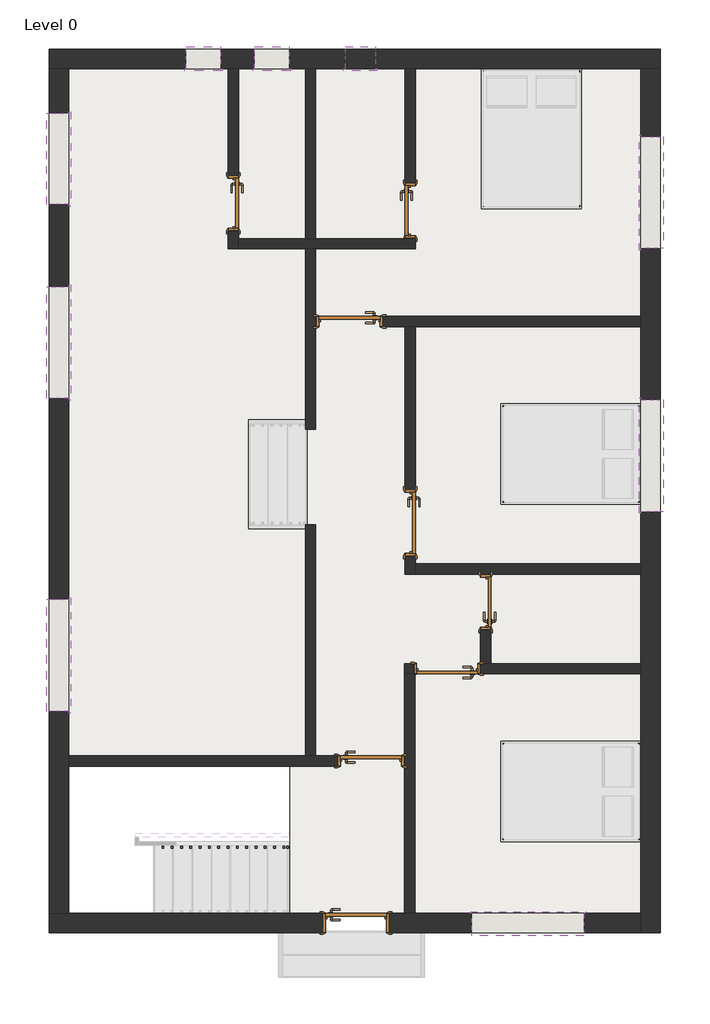
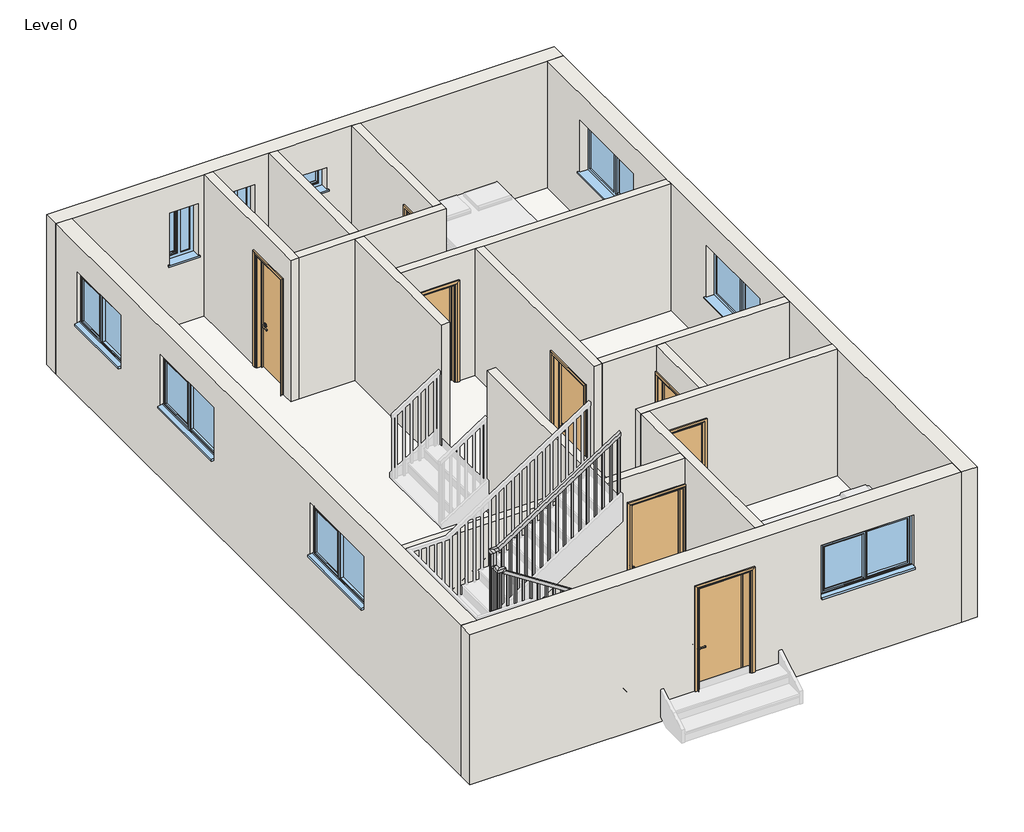
# One storey, part 1 of 2: 16 walls, 9 windows, 8 doors, 2 slabs, 1 railing.
"""IFC4 building model written with IfcOpenShell, lengths in millimetres."""

from ifc_helpers import new_model, si_unit, frame, origin, origin_with_axes, place, context, project, spatial, polyline, outline, extrude, faceted_brep, transform, mapped, element, save
from components import doors_intsgl_d1_661c03a1, doors_intsgl_d1_9c7e8c97, doors_intsgl_d1_8eed65bb, doors_intsgl_d2_f1ce814f, doors_intsgl_d2_e5ed4415, windows_dbl_plain_w1_1500_219ff321, windows_dbl_plain_w2_1220_793197e7, windows_dbl_plain_w3_460_956a2ca0, windows_sgl_plain_400mm_a5a4ca73

model = new_model("IFC4")

# Units and contexts
model_context = context("Model", 3, world=origin())
ifc_project = project(units=[si_unit("LENGTHUNIT", "METRE", prefix="MILLI")], contexts=[model_context])

# Site, building, storey
site = spatial("IfcSite", under=ifc_project)
building = spatial("IfcBuilding", under=site)
storey = spatial("IfcBuildingStorey", under=building, Name="Level 0", Elevation=0.0)

# Doors
placement = place(None, origin())
doors_intsgl_d1_shape = doors_intsgl_d1_661c03a1(model_context)
element("IfcDoor", 1, ObjectType="Doors_IntSgl : D1", at=placement, inside=storey, context=model_context, shape_type="MappedRepresentation", body=[
    mapped(doors_intsgl_d1_shape, transform((-4659.8904087, 8516.998858, 0.0), x_axis=(-1.0, 0.0, 0.0), y_axis=(0.0, -1.0, 0.0), z_axis=(0.0, 0.0, 1.0))),
])
doors_intsgl_d1_2_shape = doors_intsgl_d1_9c7e8c97(model_context)
element("IfcDoor", 2, ObjectType="Doors_IntSgl : D1", at=placement, inside=storey, context=model_context, shape_type="MappedRepresentation", body=[
    mapped(doors_intsgl_d1_2_shape, transform((-3844.8904087, 5816.998858, 0.0), x_axis=(0.0, -1.0, 0.0), y_axis=(1.0, 0.0, 0.0), z_axis=(0.0, 0.0, 1.0))),
])
element("IfcDoor", 3, ObjectType="Doors_IntSgl : D1", at=placement, inside=storey, context=model_context, shape_type="MappedRepresentation", body=[
    mapped(doors_intsgl_d1_2_shape, transform((-3349.8904087, 3856.998858, 0.0), x_axis=(-1.0, 0.0, 0.0), y_axis=(0.0, -1.0, 0.0), z_axis=(0.0, 0.0, 1.0))),
])
element("IfcDoor", 4, ObjectType="Doors_IntSgl : D1", at=placement, inside=storey, context=model_context, shape_type="MappedRepresentation", body=[
    mapped(doors_intsgl_d1_2_shape, transform((-4374.8904087, 2616.998858, 0.0), x_axis=(1.0, 0.0, 0.0), y_axis=(0.0, 1.0, 0.0), z_axis=(0.0, 0.0, 1.0))),
])
doors_intsgl_d1_3_shape = doors_intsgl_d1_8eed65bb(model_context)
element("IfcDoor", 5, ObjectType="Doors_IntSgl : D1", at=placement, inside=storey, context=model_context, shape_type="MappedRepresentation", body=[
    mapped(doors_intsgl_d1_3_shape, transform((-4574.8904087, 442.7642586, 0.0), x_axis=(1.0, 0.0, 0.0), y_axis=(0.0, 1.0, 0.0), z_axis=(0.0, 0.0, 1.0))),
])
doors_intsgl_d2_shape = doors_intsgl_d2_f1ce814f(model_context)
element("IfcDoor", 6, ObjectType="Doors_IntSgl : D2", at=placement, inside=storey, context=model_context, shape_type="MappedRepresentation", body=[
    mapped(doors_intsgl_d2_shape, transform((-3844.8904087, 10007.7642586, 0.0), x_axis=(0.0, -1.0, 0.0), y_axis=(1.0, 0.0, 0.0), z_axis=(0.0, 0.0, 1.0))),
])
element("IfcDoor", 7, ObjectType="Doors_IntSgl : D2", at=placement, inside=storey, context=model_context, shape_type="MappedRepresentation", body=[
    mapped(doors_intsgl_d2_shape, transform((-2829.8904087, 4751.998858, 0.0), x_axis=(0.0, 1.0, 0.0), y_axis=(-1.0, 0.0, 0.0), z_axis=(0.0, 0.0, 1.0))),
])
doors_intsgl_d2_2_shape = doors_intsgl_d2_e5ed4415(model_context)
element("IfcDoor", 8, ObjectType="Doors_IntSgl : D2", at=placement, inside=storey, context=model_context, shape_type="MappedRepresentation", body=[
    mapped(doors_intsgl_d2_2_shape, transform((-6224.8904087, 10107.7642586, 0.0), x_axis=(0.0, -1.0, 0.0), y_axis=(1.0, 0.0, 0.0), z_axis=(0.0, 0.0, 1.0))),
])

# Railing
element("IfcRailing", 9, ObjectType="1100mm", at=placement, inside=storey, context=model_context, shape_type="SolidModel", body=[
    faceted_brep([(-5481.4951322, 1436.1182736, 1266.6666667), (-5481.4951322, 1436.1182736, 1207.1072108), (-5481.4951322, 1486.1182736, 1207.1072108), (-5481.4951322, 1486.1182736, 1266.6666667), (-7466.8951322, 1436.1182736, 2551.7152104), (-7516.8951322, 1436.1182736, 2524.518214), (-7516.8951322, 1486.1182736, 2524.518214), (-7466.8951322, 1486.1182736, 2551.7152104), (-7466.8951322, 1436.1182736, 2600.0), (-7516.8951322, 1436.1182736, 2550.0), (-7516.8951322, 1486.1182736, 2550.0), (-7466.8951322, 1486.1182736, 2600.0), (-7591.8951322, 1436.1182736, 2600.0), (-7591.8951322, 1436.1182736, 2550.0), (-7541.8951322, 1486.1182736, 2550.0), (-7541.8951322, 1486.1182736, 2600.0), (-7591.8951322, 1561.1182736, 2600.0), (-7591.8951322, 1561.1182736, 2550.0), (-7541.8951322, 1561.1182736, 2550.0), (-7541.8951322, 1561.1182736, 2600.0), (-7591.8951322, 1571.9182736, 2600.0), (-7591.8951322, 1621.9182736, 2550.0), (-7541.8951322, 1621.9182736, 2550.0), (-7541.8951322, 1571.9182736, 2600.0), (-7591.8951322, 1571.9182736, 2814.9514563), (-7591.8951322, 1621.9182736, 2764.9514563), (-7541.8951322, 1621.9182736, 2764.9514563), (-7541.8951322, 1571.9182736, 2814.9514563), (-7591.8951322, 1696.9182736, 2814.9514563), (-7591.8951322, 1696.9182736, 2764.9514563), (-7541.8951322, 1646.9182736, 2764.9514563), (-7541.8951322, 1646.9182736, 2814.9514563), (-7466.8951322, 1696.9182736, 2814.9514563), (-7452.1257728, 1696.9182736, 2764.9514563), (-7452.1257728, 1646.9182736, 2764.9514563), (-7466.8951322, 1646.9182736, 2814.9514563), (-5481.4951322, 1696.9182736, 4100.0), (-5481.4951322, 1646.9182736, 4100.0), (-5481.4951322, 1646.9182736, 4040.4405441), (-5481.4951322, 1696.9182736, 4040.4405441)], [[[0, 1, 2, 3]], [[1, 0, 4, 5]], [[2, 1, 5, 6]], [[3, 2, 6, 7]], [[0, 3, 7, 4]], [[5, 4, 8, 9]], [[6, 5, 9, 10]], [[7, 6, 10, 11]], [[4, 7, 11, 8]], [[9, 8, 12, 13]], [[10, 9, 13, 14]], [[11, 10, 14, 15]], [[8, 11, 15, 12]], [[13, 12, 16, 17]], [[14, 13, 17, 18]], [[15, 14, 18, 19]], [[12, 15, 19, 16]], [[17, 16, 20, 21]], [[18, 17, 21, 22]], [[19, 18, 22, 23]], [[16, 19, 23, 20]], [[21, 20, 24, 25]], [[22, 21, 25, 26]], [[23, 22, 26, 27]], [[20, 23, 27, 24]], [[25, 24, 28, 29]], [[26, 25, 29, 30]], [[27, 26, 30, 31]], [[24, 27, 31, 28]], [[29, 28, 32, 33]], [[30, 29, 33, 34]], [[31, 30, 34, 35]], [[28, 31, 35, 32]], [[36, 37, 38, 39]], [[33, 32, 36, 39]], [[34, 33, 39, 38]], [[35, 34, 38, 37]], [[32, 35, 37, 36]]]),
    extrude(outline(polyline([(4017.5279227, -5516.8951322), (2833.3333333, -5516.8951322), (2833.3333333, -5491.8951322), (4033.7091525, -5491.8951322), (4017.5279227, -5516.8951322)])), frame((0.0, 1659.4182736, 0.0), z_axis=(0.0, 1.0, 0.0), x_axis=(0.0, 0.0, 1.0)), (0.0, 0.0, 1.0), 25.0),
    extrude(outline(polyline([(3936.6217739, -5641.8951322), (2833.3333333, -5641.8951322), (2833.3333333, -5616.8951322), (3952.8030036, -5616.8951322), (3936.6217739, -5641.8951322)])), frame((0.0, 1659.4182736, 0.0), z_axis=(0.0, 1.0, 0.0), x_axis=(0.0, 0.0, 1.0)), (0.0, 0.0, 1.0), 25.0),
    extrude(outline(polyline([(3855.715625, -5766.8951322), (2833.3333333, -5766.8951322), (2833.3333333, -5741.8951322), (3871.8968548, -5741.8951322), (3855.715625, -5766.8951322)])), frame((0.0, 1659.4182736, 0.0), z_axis=(0.0, 1.0, 0.0), x_axis=(0.0, 0.0, 1.0)), (0.0, 0.0, 1.0), 25.0),
    extrude(outline(polyline([(3774.8094761, -5891.8951322), (2666.6666667, -5891.8951322), (2666.6666667, -5866.8951322), (3790.9907059, -5866.8951322), (3774.8094761, -5891.8951322)])), frame((0.0, 1659.4182736, 0.0), z_axis=(0.0, 1.0, 0.0), x_axis=(0.0, 0.0, 1.0)), (0.0, 0.0, 1.0), 25.0),
    extrude(outline(polyline([(3693.9033273, -6016.8951322), (2500.0, -6016.8951322), (2500.0, -5991.8951322), (3710.084557, -5991.8951322), (3693.9033273, -6016.8951322)])), frame((0.0, 1659.4182736, 0.0), z_axis=(0.0, 1.0, 0.0), x_axis=(0.0, 0.0, 1.0)), (0.0, 0.0, 1.0), 25.0),
    extrude(outline(polyline([(3612.9971784, -6141.8951322), (2500.0, -6141.8951322), (2500.0, -6116.8951322), (3629.1784082, -6116.8951322), (3612.9971784, -6141.8951322)])), frame((0.0, 1659.4182736, 0.0), z_axis=(0.0, 1.0, 0.0), x_axis=(0.0, 0.0, 1.0)), (0.0, 0.0, 1.0), 25.0),
    extrude(outline(polyline([(3532.0910295, -6266.8951322), (2500.0, -6266.8951322), (2500.0, -6241.8951322), (3548.2722593, -6241.8951322), (3532.0910295, -6266.8951322)])), frame((0.0, 1659.4182736, 0.0), z_axis=(0.0, 1.0, 0.0), x_axis=(0.0, 0.0, 1.0)), (0.0, 0.0, 1.0), 25.0),
    extrude(outline(polyline([(3451.1848807, -6391.8951322), (2333.3333333, -6391.8951322), (2333.3333333, -6366.8951322), (3467.3661104, -6366.8951322), (3451.1848807, -6391.8951322)])), frame((0.0, 1659.4182736, 0.0), z_axis=(0.0, 1.0, 0.0), x_axis=(0.0, 0.0, 1.0)), (0.0, 0.0, 1.0), 25.0),
    extrude(outline(polyline([(3370.2787318, -6516.8951322), (2333.3333333, -6516.8951322), (2333.3333333, -6491.8951322), (3386.4599616, -6491.8951322), (3370.2787318, -6516.8951322)])), frame((0.0, 1659.4182736, 0.0), z_axis=(0.0, 1.0, 0.0), x_axis=(0.0, 0.0, 1.0)), (0.0, 0.0, 1.0), 25.0),
    extrude(outline(polyline([(3289.3725829, -6641.8951322), (2166.6666667, -6641.8951322), (2166.6666667, -6616.8951322), (3305.5538127, -6616.8951322), (3289.3725829, -6641.8951322)])), frame((0.0, 1659.4182736, 0.0), z_axis=(0.0, 1.0, 0.0), x_axis=(0.0, 0.0, 1.0)), (0.0, 0.0, 1.0), 25.0),
    extrude(outline(polyline([(3208.4664341, -6766.8951322), (2166.6666667, -6766.8951322), (2166.6666667, -6741.8951322), (3224.6476638, -6741.8951322), (3208.4664341, -6766.8951322)])), frame((0.0, 1659.4182736, 0.0), z_axis=(0.0, 1.0, 0.0), x_axis=(0.0, 0.0, 1.0)), (0.0, 0.0, 1.0), 25.0),
    extrude(outline(polyline([(3127.5602852, -6891.8951322), (2000.0, -6891.8951322), (2000.0, -6866.8951322), (3143.741515, -6866.8951322), (3127.5602852, -6891.8951322)])), frame((0.0, 1659.4182736, 0.0), z_axis=(0.0, 1.0, 0.0), x_axis=(0.0, 0.0, 1.0)), (0.0, 0.0, 1.0), 25.0),
    extrude(outline(polyline([(3046.6541363, -7016.8951322), (2000.0, -7016.8951322), (2000.0, -6991.8951322), (3062.8353661, -6991.8951322), (3046.6541363, -7016.8951322)])), frame((0.0, 1659.4182736, 0.0), z_axis=(0.0, 1.0, 0.0), x_axis=(0.0, 0.0, 1.0)), (0.0, 0.0, 1.0), 25.0),
    extrude(outline(polyline([(2965.7479875, -7141.8951322), (1833.3333333, -7141.8951322), (1833.3333333, -7116.8951322), (2981.9292172, -7116.8951322), (2965.7479875, -7141.8951322)])), frame((0.0, 1659.4182736, 0.0), z_axis=(0.0, 1.0, 0.0), x_axis=(0.0, 0.0, 1.0)), (0.0, 0.0, 1.0), 25.0),
    extrude(outline(polyline([(2884.8418386, -7266.8951322), (1833.3333333, -7266.8951322), (1833.3333333, -7241.8951322), (2901.0230684, -7241.8951322), (2884.8418386, -7266.8951322)])), frame((0.0, 1659.4182736, 0.0), z_axis=(0.0, 1.0, 0.0), x_axis=(0.0, 0.0, 1.0)), (0.0, 0.0, 1.0), 25.0),
    extrude(outline(polyline([(2803.9356897, -7391.8951322), (1666.6666667, -7391.8951322), (1666.6666667, -7366.8951322), (2820.1169195, -7366.8951322), (2803.9356897, -7391.8951322)])), frame((0.0, 1659.4182736, 0.0), z_axis=(0.0, 1.0, 0.0), x_axis=(0.0, 0.0, 1.0)), (0.0, 0.0, 1.0), 25.0),
    extrude(outline(polyline([(-7516.8951322, 1659.4182736), (-7516.8951322, 1684.4182736), (-7491.8951322, 1684.4182736), (-7491.8951322, 1659.4182736), (-7516.8951322, 1659.4182736)])), frame((0.0, 0.0, 1666.6666667), z_axis=(0.0, 0.0, 1.0), x_axis=(1.0, 0.0, 0.0)), (0.0, 0.0, 1.0), 1098.2847896),
    extrude(outline(polyline([(-7554.3951322, 1636.1182736), (-7579.3951322, 1636.1182736), (-7579.3951322, 1661.1182736), (-7554.3951322, 1661.1182736), (-7554.3951322, 1636.1182736)])), frame((0.0, 0.0, 1500.0), z_axis=(0.0, 0.0, 1.0), x_axis=(1.0, 0.0, 0.0)), (0.0, 0.0, 1.0), 1264.9514563),
    extrude(outline(polyline([(-7554.3951322, 1511.1182736), (-7579.3951322, 1511.1182736), (-7579.3951322, 1536.1182736), (-7554.3951322, 1536.1182736), (-7554.3951322, 1511.1182736)])), frame((0.0, 0.0, 1500.0), z_axis=(0.0, 0.0, 1.0), x_axis=(1.0, 0.0, 0.0)), (0.0, 0.0, 1.0), 1050.0),
    extrude(outline(polyline([(-7531.4951322, 1473.6182736), (-7531.4951322, 1448.6182736), (-7556.4951322, 1448.6182736), (-7556.4951322, 1473.6182736), (-7531.4951322, 1473.6182736)])), frame((0.0, 0.0, 1500.0), z_axis=(0.0, 0.0, 1.0), x_axis=(1.0, 0.0, 0.0)), (0.0, 0.0, 1.0), 1050.0),
    extrude(outline(polyline([(1333.3333333, -7406.4951322), (2453.0619033, -7406.4951322), (2469.2431331, -7431.4951322), (1333.3333333, -7431.4951322), (1333.3333333, -7406.4951322)])), frame((0.0, 1448.6182736, 0.0), z_axis=(0.0, 1.0, 0.0), x_axis=(0.0, 0.0, 1.0)), (0.0, 0.0, 1.0), 25.0),
    extrude(outline(polyline([(1333.3333333, -7281.4951322), (2372.1557544, -7281.4951322), (2388.3369842, -7306.4951322), (1333.3333333, -7306.4951322), (1333.3333333, -7281.4951322)])), frame((0.0, 1448.6182736, 0.0), z_axis=(0.0, 1.0, 0.0), x_axis=(0.0, 0.0, 1.0)), (0.0, 0.0, 1.0), 25.0),
    extrude(outline(polyline([(1166.6666667, -7156.4951322), (2291.2496056, -7156.4951322), (2307.4308354, -7181.4951322), (1166.6666667, -7181.4951322), (1166.6666667, -7156.4951322)])), frame((0.0, 1448.6182736, 0.0), z_axis=(0.0, 1.0, 0.0), x_axis=(0.0, 0.0, 1.0)), (0.0, 0.0, 1.0), 25.0),
    extrude(outline(polyline([(1166.6666667, -7031.4951322), (2210.3434567, -7031.4951322), (2226.5246865, -7056.4951322), (1166.6666667, -7056.4951322), (1166.6666667, -7031.4951322)])), frame((0.0, 1448.6182736, 0.0), z_axis=(0.0, 1.0, 0.0), x_axis=(0.0, 0.0, 1.0)), (0.0, 0.0, 1.0), 25.0),
    extrude(outline(polyline([(1000.0, -6906.4951322), (2129.4373078, -6906.4951322), (2145.6185376, -6931.4951322), (1000.0, -6931.4951322), (1000.0, -6906.4951322)])), frame((0.0, 1448.6182736, 0.0), z_axis=(0.0, 1.0, 0.0), x_axis=(0.0, 0.0, 1.0)), (0.0, 0.0, 1.0), 25.0),
    extrude(outline(polyline([(1000.0, -6781.4951322), (2048.531159, -6781.4951322), (2064.7123888, -6806.4951322), (1000.0, -6806.4951322), (1000.0, -6781.4951322)])), frame((0.0, 1448.6182736, 0.0), z_axis=(0.0, 1.0, 0.0), x_axis=(0.0, 0.0, 1.0)), (0.0, 0.0, 1.0), 25.0),
    extrude(outline(polyline([(833.3333333, -6656.4951322), (1967.6250101, -6656.4951322), (1983.8062399, -6681.4951322), (833.3333333, -6681.4951322), (833.3333333, -6656.4951322)])), frame((0.0, 1448.6182736, 0.0), z_axis=(0.0, 1.0, 0.0), x_axis=(0.0, 0.0, 1.0)), (0.0, 0.0, 1.0), 25.0),
    extrude(outline(polyline([(833.3333333, -6531.4951322), (1886.7188612, -6531.4951322), (1902.900091, -6556.4951322), (833.3333333, -6556.4951322), (833.3333333, -6531.4951322)])), frame((0.0, 1448.6182736, 0.0), z_axis=(0.0, 1.0, 0.0), x_axis=(0.0, 0.0, 1.0)), (0.0, 0.0, 1.0), 25.0),
    extrude(outline(polyline([(666.6666667, -6406.4951322), (1805.8127124, -6406.4951322), (1821.9939422, -6431.4951322), (666.6666667, -6431.4951322), (666.6666667, -6406.4951322)])), frame((0.0, 1448.6182736, 0.0), z_axis=(0.0, 1.0, 0.0), x_axis=(0.0, 0.0, 1.0)), (0.0, 0.0, 1.0), 25.0),
    extrude(outline(polyline([(666.6666667, -6281.4951322), (1724.9065635, -6281.4951322), (1741.0877933, -6306.4951322), (666.6666667, -6306.4951322), (666.6666667, -6281.4951322)])), frame((0.0, 1448.6182736, 0.0), z_axis=(0.0, 1.0, 0.0), x_axis=(0.0, 0.0, 1.0)), (0.0, 0.0, 1.0), 25.0),
    extrude(outline(polyline([(500.0, -6156.4951322), (1644.0004146, -6156.4951322), (1660.1816444, -6181.4951322), (500.0, -6181.4951322), (500.0, -6156.4951322)])), frame((0.0, 1448.6182736, 0.0), z_axis=(0.0, 1.0, 0.0), x_axis=(0.0, 0.0, 1.0)), (0.0, 0.0, 1.0), 25.0),
    extrude(outline(polyline([(500.0, -6031.4951322), (1563.0942658, -6031.4951322), (1579.2754955, -6056.4951322), (500.0, -6056.4951322), (500.0, -6031.4951322)])), frame((0.0, 1448.6182736, 0.0), z_axis=(0.0, 1.0, 0.0), x_axis=(0.0, 0.0, 1.0)), (0.0, 0.0, 1.0), 25.0),
    extrude(outline(polyline([(333.3333333, -5906.4951322), (1482.1881169, -5906.4951322), (1498.3693467, -5931.4951322), (333.3333333, -5931.4951322), (333.3333333, -5906.4951322)])), frame((0.0, 1448.6182736, 0.0), z_axis=(0.0, 1.0, 0.0), x_axis=(0.0, 0.0, 1.0)), (0.0, 0.0, 1.0), 25.0),
    extrude(outline(polyline([(333.3333333, -5781.4951322), (1401.281968, -5781.4951322), (1417.4631978, -5806.4951322), (333.3333333, -5806.4951322), (333.3333333, -5781.4951322)])), frame((0.0, 1448.6182736, 0.0), z_axis=(0.0, 1.0, 0.0), x_axis=(0.0, 0.0, 1.0)), (0.0, 0.0, 1.0), 25.0),
    extrude(outline(polyline([(166.6666667, -5656.4951322), (1320.3758192, -5656.4951322), (1336.5570489, -5681.4951322), (166.6666667, -5681.4951322), (166.6666667, -5656.4951322)])), frame((0.0, 1448.6182736, 0.0), z_axis=(0.0, 1.0, 0.0), x_axis=(0.0, 0.0, 1.0)), (0.0, 0.0, 1.0), 25.0),
    extrude(outline(polyline([(166.6666667, -5531.4951322), (1239.4696703, -5531.4951322), (1255.6509001, -5556.4951322), (166.6666667, -5556.4951322), (166.6666667, -5531.4951322)])), frame((0.0, 1448.6182736, 0.0), z_axis=(0.0, 1.0, 0.0), x_axis=(0.0, 0.0, 1.0)), (0.0, 0.0, 1.0), 25.0),
    extrude(outline(polyline([(-7554.3951322, 1659.4182736), (-7579.3951322, 1659.4182736), (-7579.3951322, 1684.4182736), (-7554.3951322, 1684.4182736), (-7554.3951322, 1659.4182736)])), frame((0.0, 0.0, 1500.0), z_axis=(0.0, 0.0, 1.0), x_axis=(1.0, 0.0, 0.0)), (0.0, 0.0, 1.0), 1264.9514563),
    extrude(outline(polyline([(-7554.3951322, 1473.6182736), (-7554.3951322, 1448.6182736), (-7579.3951322, 1448.6182736), (-7579.3951322, 1473.6182736), (-7554.3951322, 1473.6182736)])), frame((0.0, 0.0, 1500.0), z_axis=(0.0, 0.0, 1.0), x_axis=(1.0, 0.0, 0.0)), (0.0, 0.0, 1.0), 1050.0),
    extrude(outline(polyline([(4024.2593143, -5506.4951322), (2833.3333333, -5506.4951322), (2833.3333333, -5481.4951322), (4040.4405441, -5481.4951322), (4024.2593143, -5506.4951322)])), frame((0.0, 1659.4182736, 0.0), z_axis=(0.0, 1.0, 0.0), x_axis=(0.0, 0.0, 1.0)), (0.0, 0.0, 1.0), 25.0),
    extrude(outline(polyline([(166.6666667, -5481.4951322), (1207.1072108, -5481.4951322), (1223.2884405, -5506.4951322), (166.6666667, -5506.4951322), (166.6666667, -5481.4951322)])), frame((0.0, 1448.6182736, 0.0), z_axis=(0.0, 1.0, 0.0), x_axis=(0.0, 0.0, 1.0)), (0.0, 0.0, 1.0), 25.0),
])

# Slabs
element("IfcSlab", 10, ObjectType="FLOOR 150MM", at=placement, inside=storey, context=model_context, shape_type="SweptSolid", body=[
    extrude(outline(polyline([(-744.8904087, 11912.7642586), (-744.8904087, 572.7642586), (-5458.9951322, 572.7642586), (-5458.9951322, 2546.998858), (-5254.8904087, 2546.998858), (-5254.8904087, 11912.7642586), (-744.8904087, 11912.7642586)])), frame((0.0, 0.0, 250.0), z_axis=(0.0, 0.0, 1.0), x_axis=(1.0, 0.0, 0.0)), (0.0, 0.0, 1.0), 150.0),
])
element("IfcSlab", 11, ObjectType="FLOOR 150MM", at=placement, inside=storey, context=model_context, shape_type="SweptSolid", body=[
    extrude(outline(polyline([(-5254.8904087, 11912.7642586), (-5254.8904087, 2686.998858), (-8434.8904087, 2686.998858), (-8434.8904087, 11912.7642586), (-5254.8904087, 11912.7642586)])), origin_with_axes(), (0.0, 0.0, 1.0), 150.0),
])

# Walls
element("IfcWall", 12, at=placement, inside=storey, context=model_context, shape_type="Brep", body=[
    faceted_brep([(-8694.8904087, 11912.7642586, 0.0), (-8434.8904087, 11912.7642586, 0.0), (-6294.8904087, 11912.7642586, 0.0), (-6154.8904087, 11912.7642586, 0.0), (-5254.8904087, 11912.7642586, 0.0), (-5114.8904087, 11912.7642586, 0.0), (-3914.8904087, 11912.7642586, 0.0), (-3774.8904087, 11912.7642586, 0.0), (-744.8904087, 11912.7642586, 0.0), (-484.8904087, 11912.7642586, 0.0), (-484.8904087, 11912.7642586, 2570.0), (-744.8904087, 11912.7642586, 2570.0), (-3774.8904087, 11912.7642586, 2570.0), (-3914.8904087, 11912.7642586, 2570.0), (-5114.8904087, 11912.7642586, 2570.0), (-5254.8904087, 11912.7642586, 2570.0), (-6154.8904087, 11912.7642586, 2570.0), (-6294.8904087, 11912.7642586, 2570.0), (-8434.8904087, 11912.7642586, 2570.0), (-8694.8904087, 11912.7642586, 2570.0), (-6394.8904087, 11912.7642586, 2110.0), (-6394.8904087, 11912.7642586, 1200.0), (-6854.8904087, 11912.7642586, 1200.0), (-6854.8904087, 11912.7642586, 2110.0), (-5474.8904087, 11912.7642586, 2110.0), (-5474.8904087, 11912.7642586, 1200.0), (-5934.8904087, 11912.7642586, 1200.0), (-5934.8904087, 11912.7642586, 2110.0), (-4314.8904087, 11912.7642586, 2000.0), (-4314.8904087, 11912.7642586, 1600.0), (-4714.8904087, 11912.7642586, 1600.0), (-4714.8904087, 11912.7642586, 2000.0), (-484.8904087, 12172.7642586, 0.0), (-8694.8904087, 12172.7642586, 0.0), (-8694.8904087, 12172.7642586, 2570.0), (-484.8904087, 12172.7642586, 2570.0), (-6394.8904087, 12172.7642586, 1200.0), (-6394.8904087, 12172.7642586, 2110.0), (-6854.8904087, 12172.7642586, 2110.0), (-6854.8904087, 12172.7642586, 1200.0), (-5474.8904087, 12172.7642586, 1200.0), (-5474.8904087, 12172.7642586, 2110.0), (-5934.8904087, 12172.7642586, 2110.0), (-5934.8904087, 12172.7642586, 1200.0), (-4314.8904087, 12172.7642586, 1600.0), (-4314.8904087, 12172.7642586, 2000.0), (-4714.8904087, 12172.7642586, 2000.0), (-4714.8904087, 12172.7642586, 1600.0)], [[[0, 1, 2, 3, 4, 5, 6, 7, 8, 9, 10, 11, 12, 13, 14, 15, 16, 17, 18, 19], [20, 21, 22, 23], [24, 25, 26, 27], [28, 29, 30, 31]], [[32, 33, 34, 35], [36, 37, 38, 39], [40, 41, 42, 43], [44, 45, 46, 47]], [[9, 8, 7, 6, 5, 4, 3, 2, 1, 0, 33, 32]], [[10, 9, 32, 35]], [[0, 19, 34, 33]], [[19, 18, 17, 16, 15, 14, 13, 12, 11, 10, 35, 34]], [[21, 20, 37, 36]], [[22, 21, 36, 39]], [[23, 22, 39, 38]], [[20, 23, 38, 37]], [[25, 24, 41, 40]], [[26, 25, 40, 43]], [[27, 26, 43, 42]], [[24, 27, 42, 41]], [[28, 45, 44, 29]], [[29, 44, 47, 30]], [[30, 47, 46, 31]], [[45, 28, 31, 46]]]),
])
element("IfcWall", 13, at=placement, inside=storey, context=model_context, shape_type="Brep", body=[
    faceted_brep([(-744.8904087, 11912.7642586, 0.0), (-744.8904087, 8586.998858, 0.0), (-744.8904087, 8446.998858, 0.0), (-744.8904087, 5266.998858, 0.0), (-744.8904087, 5126.998858, 0.0), (-744.8904087, 3926.998858, 0.0), (-744.8904087, 3786.998858, 0.0), (-744.8904087, 572.7642586, 0.0), (-744.8904087, 312.7642586, 0.0), (-744.8904087, 312.7642586, 2570.0), (-744.8904087, 572.7642586, 2570.0), (-744.8904087, 3786.998858, 2570.0), (-744.8904087, 3926.998858, 2570.0), (-744.8904087, 5126.998858, 2570.0), (-744.8904087, 5266.998858, 2570.0), (-744.8904087, 8446.998858, 2570.0), (-744.8904087, 8586.998858, 2570.0), (-744.8904087, 11912.7642586, 2570.0), (-744.8904087, 10999.8815583, 2110.0), (-744.8904087, 9499.8815583, 2110.0), (-744.8904087, 9499.8815583, 1200.0), (-744.8904087, 10999.8815583, 1200.0), (-744.8904087, 7466.998858, 2110.0), (-744.8904087, 5966.998858, 2110.0), (-744.8904087, 5966.998858, 1200.0), (-744.8904087, 7466.998858, 1200.0), (-484.8904087, 11912.7642586, 0.0), (-484.8904087, 11912.7642586, 2570.0), (-484.8904087, 312.7642586, 2570.0), (-484.8904087, 312.7642586, 0.0), (-484.8904087, 10999.8815583, 2110.0), (-484.8904087, 10999.8815583, 1200.0), (-484.8904087, 9499.8815583, 1200.0), (-484.8904087, 9499.8815583, 2110.0), (-484.8904087, 7466.998858, 2110.0), (-484.8904087, 7466.998858, 1200.0), (-484.8904087, 5966.998858, 1200.0), (-484.8904087, 5966.998858, 2110.0)], [[[0, 1, 2, 3, 4, 5, 6, 7, 8, 9, 10, 11, 12, 13, 14, 15, 16, 17], [18, 19, 20, 21], [22, 23, 24, 25]], [[26, 27, 28, 29], [30, 31, 32, 33], [34, 35, 36, 37]], [[8, 7, 6, 5, 4, 3, 2, 1, 0, 26, 29]], [[0, 17, 27, 26]], [[9, 8, 29, 28]], [[17, 16, 15, 14, 13, 12, 11, 10, 9, 28, 27]], [[31, 30, 18, 21]], [[32, 31, 21, 20]], [[33, 32, 20, 19]], [[30, 33, 19, 18]], [[35, 34, 22, 25]], [[36, 35, 25, 24]], [[37, 36, 24, 23]], [[34, 37, 23, 22]]]),
])
element("IfcWall", 14, at=placement, inside=storey, context=model_context, shape_type="Brep", body=[
    faceted_brep([(-744.8904087, 572.7642586, 2570.0), (-744.8904087, 572.7642586, 0.0), (-3784.8904087, 572.7642586, 0.0), (-3924.8904087, 572.7642586, 0.0), (-4124.8904087, 572.7642586, 0.0), (-4124.8904087, 572.7642586, 2100.0), (-5024.8904087, 572.7642586, 2100.0), (-5024.8904087, 572.7642586, 0.0), (-8434.8904087, 572.7642586, 0.0), (-8694.8904087, 572.7642586, 0.0), (-8694.8904087, 572.7642586, 2570.0), (-8434.8904087, 572.7642586, 2570.0), (-3924.8904087, 572.7642586, 2570.0), (-3784.8904087, 572.7642586, 2570.0), (-1514.8904087, 572.7642586, 2110.0), (-3014.8904087, 572.7642586, 2110.0), (-3014.8904087, 572.7642586, 1200.0), (-1514.8904087, 572.7642586, 1200.0), (-744.8904087, 312.7642586, 0.0), (-744.8904087, 312.7642586, 2570.0), (-8694.8904087, 312.7642586, 2570.0), (-8694.8904087, 312.7642586, 0.0), (-5024.8904087, 312.7642586, 0.0), (-5024.8904087, 312.7642586, 2100.0), (-4124.8904087, 312.7642586, 2100.0), (-4124.8904087, 312.7642586, 0.0), (-1514.8904087, 312.7642586, 2110.0), (-1514.8904087, 312.7642586, 1200.0), (-3014.8904087, 312.7642586, 1200.0), (-3014.8904087, 312.7642586, 2110.0)], [[[0, 1, 2, 3, 4, 5, 6, 7, 8, 9, 10, 11, 12, 13], [14, 15, 16, 17]], [[18, 19, 20, 21, 22, 23, 24, 25], [26, 27, 28, 29]], [[1, 18, 25, 4, 3, 2]], [[21, 9, 8, 7, 22]], [[1, 0, 19, 18]], [[10, 9, 21, 20]], [[24, 5, 4, 25]], [[5, 24, 23, 6]], [[6, 23, 22, 7]], [[0, 13, 12, 11, 10, 20, 19]], [[27, 26, 14, 17]], [[28, 27, 17, 16]], [[29, 28, 16, 15]], [[26, 29, 15, 14]]]),
])
element("IfcWall", 15, at=placement, inside=storey, context=model_context, shape_type="Brep", body=[
    faceted_brep([(-8434.8904087, 572.7642586, 0.0), (-8434.8904087, 2546.998858, 0.0), (-8434.8904087, 2686.998858, 0.0), (-8434.8904087, 11912.7642586, 0.0), (-8434.8904087, 11912.7642586, 2570.0), (-8434.8904087, 2686.998858, 2570.0), (-8434.8904087, 2546.998858, 2570.0), (-8434.8904087, 572.7642586, 2570.0), (-8434.8904087, 3286.998858, 2110.0), (-8434.8904087, 4786.998858, 2110.0), (-8434.8904087, 4786.998858, 1200.0), (-8434.8904087, 3286.998858, 1200.0), (-8434.8904087, 7486.998858, 2110.0), (-8434.8904087, 8986.998858, 2110.0), (-8434.8904087, 8986.998858, 1200.0), (-8434.8904087, 7486.998858, 1200.0), (-8434.8904087, 10092.7642586, 2110.0), (-8434.8904087, 11312.7642586, 2110.0), (-8434.8904087, 11312.7642586, 1200.0), (-8434.8904087, 10092.7642586, 1200.0), (-8694.8904087, 572.7642586, 0.0), (-8694.8904087, 572.7642586, 2570.0), (-8694.8904087, 11912.7642586, 2570.0), (-8694.8904087, 11912.7642586, 0.0), (-8694.8904087, 3286.998858, 2110.0), (-8694.8904087, 3286.998858, 1200.0), (-8694.8904087, 4786.998858, 1200.0), (-8694.8904087, 4786.998858, 2110.0), (-8694.8904087, 7486.998858, 2110.0), (-8694.8904087, 7486.998858, 1200.0), (-8694.8904087, 8986.998858, 1200.0), (-8694.8904087, 8986.998858, 2110.0), (-8694.8904087, 10092.7642586, 2110.0), (-8694.8904087, 10092.7642586, 1200.0), (-8694.8904087, 11312.7642586, 1200.0), (-8694.8904087, 11312.7642586, 2110.0)], [[[0, 1, 2, 3, 4, 5, 6, 7], [8, 9, 10, 11], [12, 13, 14, 15], [16, 17, 18, 19]], [[20, 21, 22, 23], [24, 25, 26, 27], [28, 29, 30, 31], [32, 33, 34, 35]], [[3, 2, 1, 0, 20, 23]], [[4, 3, 23, 22]], [[0, 7, 21, 20]], [[7, 6, 5, 4, 22, 21]], [[25, 24, 8, 11]], [[26, 25, 11, 10]], [[27, 26, 10, 9]], [[24, 27, 9, 8]], [[29, 28, 12, 15]], [[30, 29, 15, 14]], [[31, 30, 14, 13]], [[28, 31, 13, 12]], [[33, 32, 16, 19]], [[34, 33, 19, 18]], [[35, 34, 18, 17]], [[32, 35, 17, 16]]]),
])
element("IfcWall", 16, ObjectType="140MM INNER WALL", at=placement, inside=storey, context=model_context, shape_type="Brep", body=[
    faceted_brep([(-6294.8904087, 11912.7642586, 2570.0), (-6294.8904087, 11912.7642586, 0.0), (-6294.8904087, 10482.7642586, 0.0), (-6294.8904087, 10482.7642586, 2100.0), (-6294.8904087, 9732.7642586, 2100.0), (-6294.8904087, 9732.7642586, 0.0), (-6294.8904087, 9492.7642586, 0.0), (-6294.8904087, 9492.7642586, 2570.0), (-6154.8904087, 11912.7642586, 0.0), (-6154.8904087, 11912.7642586, 2570.0), (-6154.8904087, 9632.7642586, 2570.0), (-6154.8904087, 9492.7642586, 2570.0), (-6154.8904087, 9492.7642586, 0.0), (-6154.8904087, 9632.7642586, 0.0), (-6154.8904087, 9732.7642586, 0.0), (-6154.8904087, 9732.7642586, 2100.0), (-6154.8904087, 10482.7642586, 2100.0), (-6154.8904087, 10482.7642586, 0.0)], [[[0, 1, 2, 3, 4, 5, 6, 7]], [[8, 9, 10, 11, 12, 13, 14, 15, 16, 17]], [[1, 8, 17, 2]], [[12, 6, 5, 14, 13]], [[1, 0, 9, 8]], [[7, 6, 12, 11]], [[4, 15, 14, 5]], [[15, 4, 3, 16]], [[16, 3, 2, 17]], [[0, 7, 11, 10, 9]]]),
])
element("IfcWall", 17, ObjectType="140MM INNER WALL", at=placement, inside=storey, context=model_context, shape_type="Brep", body=[
    faceted_brep([(-6154.8904087, 9492.7642586, 0.0), (-5254.8904087, 9492.7642586, 0.0), (-5114.8904087, 9492.7642586, 0.0), (-3774.8904087, 9492.7642586, 0.0), (-3774.8904087, 9492.7642586, 2570.0), (-5114.8904087, 9492.7642586, 2570.0), (-5254.8904087, 9492.7642586, 2570.0), (-6154.8904087, 9492.7642586, 2570.0), (-6154.8904087, 9632.7642586, 0.0), (-6154.8904087, 9632.7642586, 2570.0), (-5254.8904087, 9632.7642586, 2570.0), (-5114.8904087, 9632.7642586, 2570.0), (-3914.8904087, 9632.7642586, 2570.0), (-3774.8904087, 9632.7642586, 2570.0), (-3774.8904087, 9632.7642586, 2100.0), (-3774.8904087, 9632.7642586, 0.0), (-5114.8904087, 9632.7642586, 0.0), (-5254.8904087, 9632.7642586, 0.0)], [[[0, 1, 2, 3, 4, 5, 6, 7]], [[8, 9, 10, 11, 12, 13, 14, 15, 16, 17]], [[3, 2, 1, 0, 8, 17, 16, 15]], [[0, 7, 9, 8]], [[4, 3, 15, 14, 13]], [[7, 6, 5, 4, 13, 12, 11, 10, 9]]]),
])
element("IfcWall", 18, ObjectType="140MM INNER WALL", at=placement, inside=storey, context=model_context, shape_type="SweptSolid", body=[
    extrude(outline(polyline([(11912.7642586, 2570.0), (11912.7642586, 0.0), (10382.7642586, 0.0), (10382.7642586, 2100.0), (9632.7642586, 2100.0), (9632.7642586, 2570.0), (11912.7642586, 2570.0)])), frame((-3914.8904087, 0.0, 0.0), z_axis=(1.0, 0.0, 0.0), x_axis=(0.0, 1.0, 0.0)), (0.0, 0.0, 1.0), 140.0),
])
element("IfcWall", 19, ObjectType="140MM INNER WALL", at=placement, inside=storey, context=model_context, shape_type="Brep", body=[
    faceted_brep([(-5254.8904087, 7072.7642586, 0.0), (-5254.8904087, 7072.7642586, 2570.0), (-5254.8904087, 9492.7642586, 2570.0), (-5254.8904087, 9492.7642586, 0.0), (-5114.8904087, 7072.7642586, 2570.0), (-5114.8904087, 7072.7642586, 0.0), (-5114.8904087, 8446.998858, 0.0), (-5114.8904087, 8586.998858, 0.0), (-5114.8904087, 9492.7642586, 0.0), (-5114.8904087, 9492.7642586, 2570.0), (-5114.8904087, 8586.998858, 2570.0), (-5114.8904087, 8446.998858, 2570.0)], [[[0, 1, 2, 3]], [[4, 5, 6, 7, 8, 9, 10, 11]], [[5, 0, 3, 8, 7, 6]], [[1, 0, 5, 4]], [[3, 2, 9, 8]], [[1, 4, 11, 10, 9, 2]]]),
    faceted_brep([(-5254.8904087, 11912.7642586, 2570.0), (-5254.8904087, 11912.7642586, 0.0), (-5254.8904087, 9632.7642586, 0.0), (-5254.8904087, 9632.7642586, 2570.0), (-5114.8904087, 11912.7642586, 0.0), (-5114.8904087, 11912.7642586, 2570.0), (-5114.8904087, 9632.7642586, 2570.0), (-5114.8904087, 9632.7642586, 0.0)], [[[0, 1, 2, 3]], [[4, 5, 6, 7]], [[1, 4, 7, 2]], [[1, 0, 5, 4]], [[3, 2, 7, 6]], [[5, 0, 3, 6]]]),
])
element("IfcWall", 20, ObjectType="140MM INNER WALL", at=placement, inside=storey, context=model_context, shape_type="Brep", body=[
    faceted_brep([(-744.8904087, 8446.998858, 0.0), (-744.8904087, 8446.998858, 2570.0), (-3774.8904087, 8446.998858, 2570.0), (-3914.8904087, 8446.998858, 2570.0), (-5114.8904087, 8446.998858, 2570.0), (-5114.8904087, 8446.998858, 0.0), (-5109.8904087, 8446.998858, 0.0), (-5109.8904087, 8446.998858, 2100.0), (-4209.8904087, 8446.998858, 2100.0), (-4209.8904087, 8446.998858, 0.0), (-3914.8904087, 8446.998858, 0.0), (-3774.8904087, 8446.998858, 0.0), (-744.8904087, 8586.998858, 2570.0), (-744.8904087, 8586.998858, 0.0), (-4209.8904087, 8586.998858, 0.0), (-4209.8904087, 8586.998858, 2100.0), (-5109.8904087, 8586.998858, 2100.0), (-5109.8904087, 8586.998858, 0.0), (-5114.8904087, 8586.998858, 0.0), (-5114.8904087, 8586.998858, 2570.0)], [[[0, 1, 2, 3, 4, 5, 6, 7, 8, 9, 10, 11]], [[12, 13, 14, 15, 16, 17, 18, 19]], [[13, 0, 11, 10, 9, 14]], [[5, 18, 17, 6]], [[1, 0, 13, 12]], [[5, 4, 19, 18]], [[16, 7, 6, 17]], [[7, 16, 15, 8]], [[8, 15, 14, 9]], [[4, 3, 2, 1, 12, 19]]]),
])
element("IfcWall", 21, ObjectType="140MM INNER WALL", at=placement, inside=storey, context=model_context, shape_type="Brep", body=[
    faceted_brep([(-3914.8904087, 8446.998858, 2570.0), (-3914.8904087, 8446.998858, 0.0), (-3914.8904087, 6266.998858, 0.0), (-3914.8904087, 6266.998858, 2100.0), (-3914.8904087, 5366.998858, 2100.0), (-3914.8904087, 5366.998858, 0.0), (-3914.8904087, 5126.998858, 0.0), (-3914.8904087, 5126.998858, 2570.0), (-3774.8904087, 8446.998858, 0.0), (-3774.8904087, 8446.998858, 2570.0), (-3774.8904087, 5266.998858, 2570.0), (-3774.8904087, 5126.998858, 2570.0), (-3774.8904087, 5126.998858, 0.0), (-3774.8904087, 5266.998858, 0.0), (-3774.8904087, 5366.998858, 0.0), (-3774.8904087, 5366.998858, 2100.0), (-3774.8904087, 6266.998858, 2100.0), (-3774.8904087, 6266.998858, 0.0)], [[[0, 1, 2, 3, 4, 5, 6, 7]], [[8, 9, 10, 11, 12, 13, 14, 15, 16, 17]], [[1, 8, 17, 2]], [[12, 6, 5, 14, 13]], [[1, 0, 9, 8]], [[7, 6, 12, 11]], [[4, 15, 14, 5]], [[15, 4, 3, 16]], [[16, 3, 2, 17]], [[0, 7, 11, 10, 9]]]),
])
element("IfcWall", 22, ObjectType="140MM INNER WALL", at=placement, inside=storey, context=model_context, shape_type="Brep", body=[
    faceted_brep([(-744.8904087, 5266.998858, 0.0), (-3774.8904087, 5266.998858, 0.0), (-3774.8904087, 5266.998858, 2570.0), (-744.8904087, 5266.998858, 2570.0), (-744.8904087, 5126.998858, 0.0), (-744.8904087, 5126.998858, 2570.0), (-2759.8904087, 5126.998858, 2570.0), (-2899.8904087, 5126.998858, 2570.0), (-3774.8904087, 5126.998858, 2570.0), (-3774.8904087, 5126.998858, 0.0), (-2899.8904087, 5126.998858, 0.0), (-2759.8904087, 5126.998858, 0.0)], [[[0, 1, 2, 3]], [[4, 5, 6, 7, 8, 9, 10, 11]], [[1, 0, 4, 11, 10, 9]], [[2, 1, 9, 8]], [[0, 3, 5, 4]], [[3, 2, 8, 7, 6, 5]]]),
])
element("IfcWall", 23, ObjectType="140MM INNER WALL", at=placement, inside=storey, context=model_context, shape_type="SweptSolid", body=[
    extrude(outline(polyline([(3926.998858, 0.0), (3926.998858, 2570.0), (5126.998858, 2570.0), (5126.998858, 2100.0), (4376.998858, 2100.0), (4376.998858, 0.0), (3926.998858, 0.0)])), frame((-2899.8904087, 0.0, 0.0), z_axis=(1.0, 0.0, 0.0), x_axis=(0.0, 1.0, 0.0)), (0.0, 0.0, 1.0), 140.0),
])
element("IfcWall", 24, ObjectType="140MM INNER WALL", at=placement, inside=storey, context=model_context, shape_type="Brep", body=[
    faceted_brep([(-744.8904087, 3926.998858, 2570.0), (-744.8904087, 3926.998858, 0.0), (-2759.8904087, 3926.998858, 0.0), (-2899.8904087, 3926.998858, 0.0), (-2899.8904087, 3926.998858, 2100.0), (-3799.8904087, 3926.998858, 2100.0), (-3799.8904087, 3926.998858, 0.0), (-3924.8904087, 3926.998858, 0.0), (-3924.8904087, 3926.998858, 2570.0), (-2899.8904087, 3926.998858, 2570.0), (-2759.8904087, 3926.998858, 2570.0), (-744.8904087, 3786.998858, 0.0), (-744.8904087, 3786.998858, 2570.0), (-3784.8904087, 3786.998858, 2570.0), (-3924.8904087, 3786.998858, 2570.0), (-3924.8904087, 3786.998858, 0.0), (-3799.8904087, 3786.998858, 0.0), (-3799.8904087, 3786.998858, 2100.0), (-2899.8904087, 3786.998858, 2100.0), (-2899.8904087, 3786.998858, 0.0)], [[[0, 1, 2, 3, 4, 5, 6, 7, 8, 9, 10]], [[11, 12, 13, 14, 15, 16, 17, 18, 19]], [[1, 11, 19, 3, 2]], [[15, 7, 6, 16]], [[1, 0, 12, 11]], [[8, 7, 15, 14]], [[5, 17, 16, 6]], [[17, 5, 4, 18]], [[18, 4, 3, 19]], [[0, 10, 9, 8, 14, 13, 12]]]),
])
element("IfcWall", 25, ObjectType="140MM INNER WALL", at=placement, inside=storey, context=model_context, shape_type="Brep", body=[
    faceted_brep([(-3924.8904087, 3786.998858, 0.0), (-3924.8904087, 2686.998858, 0.0), (-3924.8904087, 2546.998858, 0.0), (-3924.8904087, 572.7642586, 0.0), (-3924.8904087, 572.7642586, 2570.0), (-3924.8904087, 2546.998858, 2570.0), (-3924.8904087, 2686.998858, 2570.0), (-3924.8904087, 3786.998858, 2570.0), (-3784.8904087, 3786.998858, 0.0), (-3784.8904087, 3786.998858, 2570.0), (-3784.8904087, 572.7642586, 2570.0), (-3784.8904087, 572.7642586, 0.0)], [[[0, 1, 2, 3, 4, 5, 6, 7]], [[8, 9, 10, 11]], [[3, 2, 1, 0, 8, 11]], [[0, 7, 9, 8]], [[4, 3, 11, 10]], [[7, 6, 5, 4, 10, 9]]]),
])
element("IfcWall", 26, ObjectType="140MM INNER WALL", at=placement, inside=storey, context=model_context, shape_type="SweptSolid", body=[
    extrude(outline(polyline([(-5254.8904087, 2686.998858), (-5254.8904087, 5786.998858), (-5114.8904087, 5786.998858), (-5114.8904087, 2686.998858), (-5254.8904087, 2686.998858)])), origin_with_axes(), (0.0, 0.0, 1.0), 2570.0),
])
element("IfcWall", 27, ObjectType="140MM INNER WALL", at=placement, inside=storey, context=model_context, shape_type="Brep", body=[
    faceted_brep([(-8434.8904087, 2686.998858, 0.0), (-8434.8904087, 2686.998858, 2570.0), (-5254.8904087, 2686.998858, 2570.0), (-5114.8904087, 2686.998858, 2570.0), (-3924.8904087, 2686.998858, 2570.0), (-3924.8904087, 2686.998858, 2100.0), (-4824.8904087, 2686.998858, 2100.0), (-4824.8904087, 2686.998858, 0.0), (-5114.8904087, 2686.998858, 0.0), (-5254.8904087, 2686.998858, 0.0), (-8434.8904087, 2546.998858, 2570.0), (-8434.8904087, 2546.998858, 0.0), (-4824.8904087, 2546.998858, 0.0), (-4824.8904087, 2546.998858, 2100.0), (-3924.8904087, 2546.998858, 2100.0), (-3924.8904087, 2546.998858, 2570.0)], [[[0, 1, 2, 3, 4, 5, 6, 7, 8, 9]], [[10, 11, 12, 13, 14, 15]], [[11, 0, 9, 8, 7, 12]], [[1, 0, 11, 10]], [[4, 15, 14, 5]], [[13, 6, 5, 14]], [[6, 13, 12, 7]], [[4, 3, 2, 1, 10, 15]]]),
])

# Windows
windows_dbl_plain_w1_1500_shape = windows_dbl_plain_w1_1500_219ff321(model_context)
element("IfcWindow", 28, ObjectType="Windows_Dbl_Plain : W1 1500", at=placement, inside=storey, context=model_context, shape_type="MappedRepresentation", body=[
    mapped(windows_dbl_plain_w1_1500_shape, transform((-623.3469765, 9964.8815583, 0.0), x_axis=(0.0, -1.0, 0.0), y_axis=(1.0, 0.0, 0.0), z_axis=(0.0, 0.0, 1.0))),
])
element("IfcWindow", 29, ObjectType="Windows_Dbl_Plain : W1 1500", at=placement, inside=storey, context=model_context, shape_type="MappedRepresentation", body=[
    mapped(windows_dbl_plain_w1_1500_shape, transform((-623.3469765, 6431.998858, 0.0), x_axis=(0.0, -1.0, 0.0), y_axis=(1.0, 0.0, 0.0), z_axis=(0.0, 0.0, 1.0))),
])
element("IfcWindow", 30, ObjectType="Windows_Dbl_Plain : W1 1500", at=placement, inside=storey, context=model_context, shape_type="MappedRepresentation", body=[
    mapped(windows_dbl_plain_w1_1500_shape, transform((-2549.8904087, 451.2208264, 0.0), x_axis=(-1.0, 0.0, 0.0), y_axis=(0.0, -1.0, 0.0), z_axis=(0.0, 0.0, 1.0))),
])
element("IfcWindow", 31, ObjectType="Windows_Dbl_Plain : W1 1500", at=placement, inside=storey, context=model_context, shape_type="MappedRepresentation", body=[
    mapped(windows_dbl_plain_w1_1500_shape, transform((-8556.4338409, 4321.998858, 0.0), x_axis=(0.0, 1.0, 0.0), y_axis=(-1.0, 0.0, 0.0), z_axis=(0.0, 0.0, 1.0))),
])
element("IfcWindow", 32, ObjectType="Windows_Dbl_Plain : W1 1500", at=placement, inside=storey, context=model_context, shape_type="MappedRepresentation", body=[
    mapped(windows_dbl_plain_w1_1500_shape, transform((-8556.4338409, 8521.998858, 0.0), x_axis=(0.0, 1.0, 0.0), y_axis=(-1.0, 0.0, 0.0), z_axis=(0.0, 0.0, 1.0))),
])
windows_dbl_plain_w2_1220_shape = windows_dbl_plain_w2_1220_793197e7(model_context)
element("IfcWindow", 33, ObjectType="Windows_Dbl_Plain : W2 1220", at=placement, inside=storey, context=model_context, shape_type="MappedRepresentation", body=[
    mapped(windows_dbl_plain_w2_1220_shape, transform((-8556.4338409, 10987.7642586, 0.0), x_axis=(0.0, 1.0, 0.0), y_axis=(-1.0, 0.0, 0.0), z_axis=(0.0, 0.0, 1.0))),
])
windows_dbl_plain_w3_460_shape = windows_dbl_plain_w3_460_956a2ca0(model_context)
element("IfcWindow", 34, ObjectType="Windows_Dbl_Plain : W3 460", at=placement, inside=storey, context=model_context, shape_type="MappedRepresentation", body=[
    mapped(windows_dbl_plain_w3_460_shape, transform((-6909.8904087, 12034.3076908, 0.0), x_axis=(-1.0, 0.0, 0.0), y_axis=(0.0, -1.0, 0.0), z_axis=(0.0, 0.0, 1.0))),
])
element("IfcWindow", 35, ObjectType="Windows_Dbl_Plain : W3 460", at=placement, inside=storey, context=model_context, shape_type="MappedRepresentation", body=[
    mapped(windows_dbl_plain_w3_460_shape, transform((-5989.8904087, 12034.3076908, 0.0), x_axis=(-1.0, 0.0, 0.0), y_axis=(0.0, -1.0, 0.0), z_axis=(0.0, 0.0, 1.0))),
])
windows_sgl_plain_400mm_shape = windows_sgl_plain_400mm_a5a4ca73(model_context)
element("IfcWindow", 36, ObjectType="Windows_Sgl_Plain : 400MM", at=placement, inside=storey, context=model_context, shape_type="MappedRepresentation", body=[
    mapped(windows_sgl_plain_400mm_shape, transform((-4514.8904087, 12034.3076908, -110.0), x_axis=(-1.0, 0.0, 0.0), y_axis=(0.0, -1.0, 0.0), z_axis=(0.0, 0.0, 1.0))),
])

save(model, "model.ifc")

# Revit data of these elements
# Type "Doors_IntSgl : D1"
#   Type Mark = "46"
#   Type Comments = "Internal Single"
#   Operation = "SingleSwingRight"
#   Manufacturer = "Revit"
#   Keynote = "L20"
#   Description = "Internal Single Door"
#   Analytic Construction = "Metal"
#   UnderCut = 8 mm
#   Tolerance = 2 mm
#   Thickness = 38 mm
#   Thermal Resistance (R) = 0.270117 (m²·K)/W
#   Structural Tolerance = 8 mm
#   StopDepth = 32 mm
#   Stop Thickness = 19 mm
#   Rough Width = 900 mm
#   Rough Height = 2100 mm
#   Height to Top Lock Rail = 1000 mm
#   Heat Transfer Coefficient (U) = 3.7021 W/(m²·K)
#   Handle Z Distance = 900 mm
#   Handle X Distance = 75 mm
#   Frame Thickness = 32 mm
#   Door Panel Width = 816 mm
#   Door Panel Thickness = 38 mm
#   Door Panel Offset = 0 mm
#   Height = 2100 mm
#   Width = 900 mm
#   Door Panel Height = 2050 mm
#   Architrave Setback = 5 mm
#   Vis - Ironmongery = yes
#   Material Ironmongery = Door - Handle
#   Material Frame = Door - Frame/Mullion (1)
#   Material Door = Door - Panel
#   Material Architrave = Door - Architrave
#   Visual Light Transmittance = 0
#   Solar Heat Gain Coefficient = 0
#   Function = (empty or 0)
#   Wall Closure = (empty or 0)
# Type "Doors_IntSgl : D2"
#   Type Mark = "47"
#   Type Comments = "Internal Single"
#   Operation = "SingleSwingRight"
#   Manufacturer = "Revit"
#   Keynote = "L20"
#   Description = "Internal Single Door"
#   Analytic Construction = "Metal"
#   UnderCut = 8 mm
#   Tolerance = 2 mm
#   Thickness = 38 mm
#   Thermal Resistance (R) = 0.270117 (m²·K)/W
#   Structural Tolerance = 8 mm
#   StopDepth = 32 mm
#   Stop Thickness = 19 mm
#   Rough Width = 750 mm
#   Rough Height = 2100 mm
#   Height to Top Lock Rail = 1000 mm
#   Heat Transfer Coefficient (U) = 3.7021 W/(m²·K)
#   Handle Z Distance = 900 mm
#   Handle X Distance = 75 mm
#   Frame Thickness = 32 mm
#   Door Panel Width = 666 mm
#   Door Panel Thickness = 38 mm
#   Door Panel Offset = 0 mm
#   Height = 2100 mm
#   Width = 750 mm
#   Door Panel Height = 2050 mm
#   Architrave Setback = 5 mm
#   Vis - Ironmongery = yes
#   Material Ironmongery = Door - Handle
#   Material Frame = Door - Frame/Mullion (1)
#   Material Door = Door - Panel
#   Material Architrave = Door - Architrave
#   Visual Light Transmittance = 0
#   Solar Heat Gain Coefficient = 0
#   Function = (empty or 0)
#   Wall Closure = (empty or 0)
# Type "1100mm"
#   built-in parameter 1008612 = 0.019685 (stored number, unit not read)
#   built-in parameter 1008611 = 0.019685 (stored number, unit not read)
#   built-in parameter 1008609 = 0.902231 (stored number, unit not read)
#   built-in parameter 1008604 = 0.19685 (stored number, unit not read)
#   built-in parameter 1008603 = 0.164042 (stored number, unit not read)
#   Railing Height = 1100 mm
#   built-in parameter 1008630 = 2
#   built-in parameter 1008610 = 2
#   built-in parameter 1008608 = 1
#   built-in parameter 1008618 = Baluster_Square : 25mm
# Type "FLOOR 150MM"
#   Function = 0
#   Layers, outside or top first: 22 mm "Wood Sheathing, Chipboard" (function 5); 128 mm "Structure, Timber Joist/Rafter Layer" (function 1)
# Type
#   Keynote = "F10"
#   Layers, outside or top first: 260 mm "Brick, Common" (function 1)
# Type "140MM INNER WALL"
#   Keynote = "F10"
#   Layers, outside or top first: 140 mm "Brick, Common" (function 1)
# Type "Windows_Dbl_Plain : W1 1500"
#   Type Mark = "62"
#   Operation = "DoublePanelVertical"
#   Construction Type Id = "GSP4R"
#   Manufacturer = "Revit"
#   Keynote = "L10"
#   Analytic Construction = "1/8 in Pilkington single glazing"
#   Wrap Layers (Ext) from Ext = 102.5 mm
#   Wrap Layers (Int) from Ext = 177.5 mm
#   Window Board Projection = 25 mm
#   Window Board Extension = 25 mm
#   Visual Light Transmittance = 0.9
#   Solar Heat Gain Coefficient = 0.78
#   Rough Width = 1500 mm
#   Rough Height = 910 mm
#   Height = 910 mm
#   Width = 1500 mm
#   Heat Transfer Coefficient (U) = 3.6886 W/(m²·K)
#   Glazing Thickness = 24 mm
#   FrameOffset - External = 50 mm
#   Frame Depth = 65 mm
#   Default Head Height = 2110 mm
#   Cill Depth = 87.5 mm
#   Cavity Closer Width = 50 mm
#   Cavity Closer Offset from Ext = 102.5 mm
#   Cavity Closer Depth = 85 mm
#   Vis - Cavity Closers = yes
#   Define Thermal Properties by = 1
#   Material Trim = Window Frame
#   Material Glass = Glass
#   Material Frame = Window Frame
#   Wall Closure = (empty or 0)
# Type "Windows_Dbl_Plain : W2 1220"
#   Type Mark = "63"
#   Operation = "DoublePanelVertical"
#   Construction Type Id = "GSP4R"
#   Manufacturer = "Revit"
#   Keynote = "L10"
#   Analytic Construction = "1/8 in Pilkington single glazing"
#   Wrap Layers (Ext) from Ext = 102.5 mm
#   Wrap Layers (Int) from Ext = 177.5 mm
#   Window Board Projection = 25 mm
#   Window Board Extension = 25 mm
#   Visual Light Transmittance = 0.9
#   Solar Heat Gain Coefficient = 0.78
#   Rough Width = 1220 mm
#   Rough Height = 910 mm
#   Height = 910 mm
#   Width = 1220 mm
#   Heat Transfer Coefficient (U) = 3.6886 W/(m²·K)
#   Glazing Thickness = 24 mm
#   FrameOffset - External = 50 mm
#   Frame Depth = 65 mm
#   Default Head Height = 2110 mm
#   Cill Depth = 87.5 mm
#   Cavity Closer Width = 50 mm
#   Cavity Closer Offset from Ext = 102.5 mm
#   Cavity Closer Depth = 85 mm
#   Vis - Cavity Closers = yes
#   Define Thermal Properties by = 1
#   Material Trim = Window Frame
#   Material Glass = Glass
#   Material Frame = Window Frame
#   Wall Closure = (empty or 0)
# Type "Windows_Dbl_Plain : W3 460"
#   Type Mark = "64"
#   Operation = "DoublePanelVertical"
#   Construction Type Id = "GSP4R"
#   Manufacturer = "Revit"
#   Keynote = "L10"
#   Analytic Construction = "1/8 in Pilkington single glazing"
#   Wrap Layers (Ext) from Ext = 102.5 mm
#   Wrap Layers (Int) from Ext = 177.5 mm
#   Window Board Projection = 25 mm
#   Window Board Extension = 25 mm
#   Visual Light Transmittance = 0.9
#   Solar Heat Gain Coefficient = 0.78
#   Rough Width = 460 mm
#   Rough Height = 910 mm
#   Height = 910 mm
#   Width = 460 mm
#   Heat Transfer Coefficient (U) = 3.6886 W/(m²·K)
#   Glazing Thickness = 24 mm
#   FrameOffset - External = 50 mm
#   Frame Depth = 65 mm
#   Default Head Height = 2110 mm
#   Cill Depth = 87.5 mm
#   Cavity Closer Width = 50 mm
#   Cavity Closer Offset from Ext = 102.5 mm
#   Cavity Closer Depth = 85 mm
#   Vis - Cavity Closers = yes
#   Define Thermal Properties by = 1
#   Material Trim = Window Frame
#   Material Glass = Glass
#   Material Frame = Window Frame
#   Wall Closure = (empty or 0)
# Type "Windows_Sgl_Plain : 400MM"
#   Type Mark = "65"
#   Operation = "SinglePanel"
#   Construction Type Id = "SGL"
#   Manufacturer = "Revit"
#   Keynote = "L10"
#   Analytic Construction = "Large single-glazed windows"
#   Wrap Layers (Ext) from Ext = 102.5 mm
#   Wrap Layers (Int) from Ext = 177.5 mm
#   Window Board Projection = 25 mm
#   Window Board Extension = 25 mm
#   Visual Light Transmittance = 0.9
#   Solar Heat Gain Coefficient = 0.86
#   Rough Width = 400 mm
#   Rough Height = 400 mm
#   Height = 400 mm
#   Width = 400 mm
#   Heat Transfer Coefficient (U) = 5.5617 W/(m²·K)
#   Glazing Thickness = 24 mm
#   FrameOffset - External = 50 mm
#   Frame Depth = 65 mm
#   Default Head Height = 2110 mm
#   Cill Depth = 87.5 mm
#   Cavity Closer Width = 50 mm
#   Cavity Closer Offset from Ext = 102.5 mm
#   Cavity Closer Depth = 85 mm
#   Vis - Cavity Closers = yes
#   Define Thermal Properties by = 1
#   Material Trim = Window Frame
#   Material Glass = Glass
#   Material Frame = Window Frame
#   Wall Closure = (empty or 0)
# Elements 1, 2, 3, 4, 5 (IfcDoor, "Doors_IntSgl : D1")
#   Phase Created = New Construction
#   Materials on its faces: "Door - Architrave", "Door - Handle", "Door - Frame/Mullion (1)", "Door - Panel"
# Elements 6, 7, 8 (IfcDoor, "Doors_IntSgl : D2")
#   Phase Created = New Construction
#   Materials on its faces: "Door - Architrave", "Door - Handle", "Door - Frame/Mullion (1)", "Door - Panel"
# Element 9 (IfcRailing, "1100mm")
#   Phase Created = New Construction
# Element 10 (IfcSlab, "FLOOR 150MM")
#   Height Offset From Level = 400 mm
#   Phase Created = New Construction
#   Materials on its faces: "Structure, Timber Joist/Rafter Layer", "Wood Sheathing, Chipboard"
# Element 11 (IfcSlab, "FLOOR 150MM")
#   Height Offset From Level = 150 mm
#   Phase Created = New Construction
#   Materials on its faces: "Structure, Timber Joist/Rafter Layer", "Wood Sheathing, Chipboard"
# Elements 12, 13, 14, 15 (IfcWall)
#   Top Offset = 0 mm
#   Base Offset = 0 mm
#   wall height = 3000 mm
#   Phase Created = New Construction
#   Base Constraint = Level 0
#   Top Constraint = Level 1
#   Materials on its faces: "Brick, Common"
# Elements 16, 17, 18, 19, 20, 21, 22, 23, 24, 25, 26, 27 (IfcWall, "140MM INNER WALL")
#   Top Offset = 0 mm
#   Base Offset = 0 mm
#   wall height = 3000 mm
#   Phase Created = New Construction
#   Base Constraint = Level 0
#   Top Constraint = Level 1
#   Materials on its faces: "Brick, Common"
# Element 28 (IfcWindow, "Windows_Dbl_Plain : W1 1500")
#   Mark = "1"
#   Phase Created = New Construction
#   Materials on its faces: "Window Frame", "Glass"
# Element 29 (IfcWindow, "Windows_Dbl_Plain : W1 1500")
#   Mark = "2"
#   Phase Created = New Construction
#   Materials on its faces: "Window Frame", "Glass"
# Element 30 (IfcWindow, "Windows_Dbl_Plain : W1 1500")
#   Mark = "3"
#   Phase Created = New Construction
#   Materials on its faces: "Window Frame", "Glass"
# Element 31 (IfcWindow, "Windows_Dbl_Plain : W1 1500")
#   Mark = "4"
#   Phase Created = New Construction
#   Materials on its faces: "Window Frame", "Glass"
# Element 32 (IfcWindow, "Windows_Dbl_Plain : W1 1500")
#   Mark = "5"
#   Phase Created = New Construction
#   Materials on its faces: "Window Frame", "Glass"
# Element 33 (IfcWindow, "Windows_Dbl_Plain : W2 1220")
#   Mark = "6"
#   Phase Created = New Construction
#   Materials on its faces: "Window Frame", "Glass"
# Element 34 (IfcWindow, "Windows_Dbl_Plain : W3 460")
#   Mark = "7"
#   Phase Created = New Construction
#   Materials on its faces: "Window Frame", "Glass"
# Element 35 (IfcWindow, "Windows_Dbl_Plain : W3 460")
#   Mark = "8"
#   Phase Created = New Construction
#   Materials on its faces: "Window Frame", "Glass"
# Element 36 (IfcWindow, "Windows_Sgl_Plain : 400MM")
#   Mark = "9"
#   Phase Created = New Construction
#   Materials on its faces: "Window Frame", "Glass"
# Materials
#   "Door - Handle": colour RGB 0 0 0, transparency 0, Keynote = "P21", Cost = 0
#   "Door - Frame/Mullion (1)": class "Wood", colour RGB 212 179 113, transparency 0, Keynote = "L20", Cost = 0
